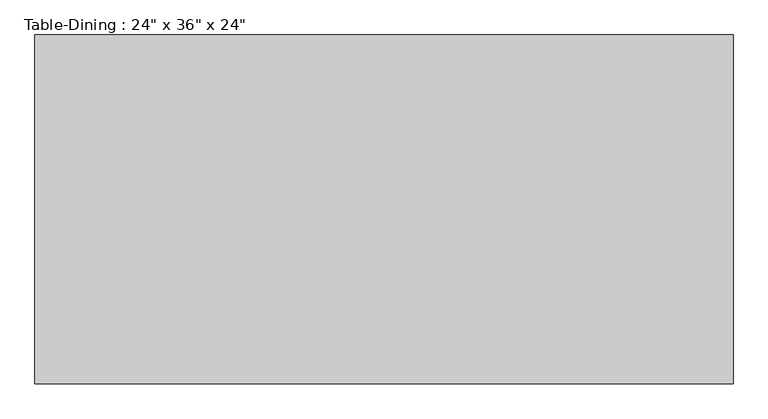
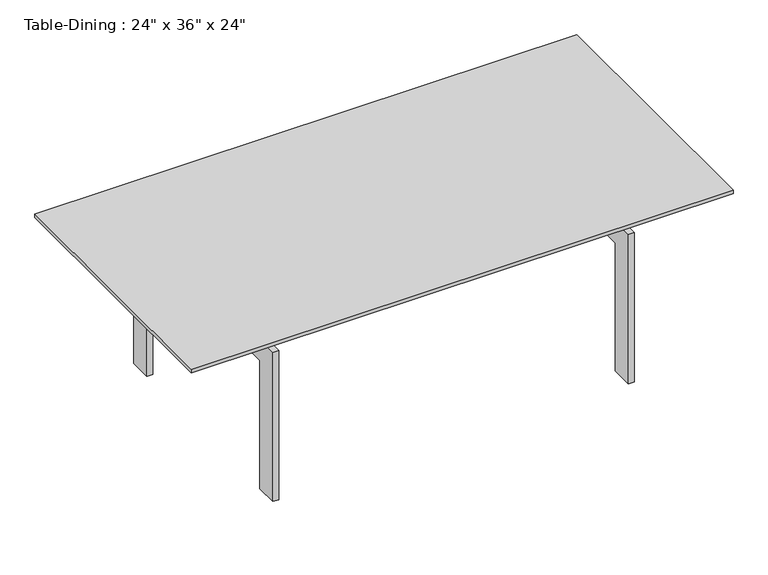
"""IFC4 building model written with IfcOpenShell, lengths in millimetres: furniture geometry."""

from ifc_helpers import new_model, si_unit, frame, origin, place, context, project, spatial, polyline, outline, extrude, source, transform, mapped, element, save


def furniture_5644571f(model_context):
    return source(origin(), model_context, "Body", "SweptSolid", [
        extrude(outline(polyline([(831.0657667, 297.7823857), (831.0657667, 272.3823857), (-794.5342333, 272.3823857), (-794.5342333, 297.7823857), (831.0657667, 297.7823857)])), frame((0.0, 0.0, 533.4), z_axis=(0.0, 0.0, 1.0), x_axis=(1.0, 0.0, 0.0)), (0.0, 0.0, 1.0), 63.5),
        extrude(outline(polyline([(831.0657667, -82.5889222), (831.0657667, -107.9889222), (-794.5342333, -107.9889222), (-794.5342333, -82.5889222), (831.0657667, -82.5889222)])), frame((0.0, 0.0, 533.4), z_axis=(0.0, 0.0, 1.0), x_axis=(1.0, 0.0, 0.0)), (0.0, 0.0, 1.0), 63.5),
        extrude(outline(polyline([(501.6110778, 0.0), (425.4110778, 0.0), (425.4110778, 457.2), (-234.9889222, 457.2), (-234.9889222, 0.0), (-311.1889222, 0.0), (-311.1889222, 533.4), (501.6110778, 533.4), (501.6110778, 0.0)])), frame((608.8157667, 0.0, 0.0), z_axis=(1.0, 0.0, 0.0), x_axis=(0.0, 1.0, 0.0)), (0.0, 0.0, 1.0), 19.05),
        extrude(outline(polyline([(501.6110778, 533.4), (501.6110778, 0.0), (425.4110778, 0.0), (425.4110778, 457.2), (-234.9889222, 457.2), (-234.9889222, 0.0), (-311.1889222, 0.0), (-311.1889222, 533.4), (501.6110778, 533.4)])), frame((-591.3342333, 0.0, 0.0), z_axis=(1.0, 0.0, 0.0), x_axis=(0.0, 1.0, 0.0)), (0.0, 0.0, 1.0), 19.05),
        extrude(outline(polyline([(932.6657667, 552.4110778), (932.6657667, -361.9889222), (-896.1342333, -361.9889222), (-896.1342333, 552.4110778), (932.6657667, 552.4110778)])), frame((0.0, 0.0, 596.9), z_axis=(0.0, 0.0, 1.0), x_axis=(1.0, 0.0, 0.0)), (0.0, 0.0, 1.0), 12.7),
    ])


if __name__ == "__main__":
    model = new_model("IFC4")
    model_context = context("Model", 3, world=origin())
    ifc_project = project(units=[si_unit("LENGTHUNIT", "METRE", prefix="MILLI")], contexts=[model_context])
    site = spatial("IfcSite", under=ifc_project)
    building = spatial("IfcBuilding", under=site)
    placement = place(None, origin())
    furniture_shape = furniture_5644571f(model_context)
    element("IfcFurniture", 1, ObjectType="Table-Dining : 24\" x 36\" x 24\"", at=placement, inside=building, context=model_context, shape_type="MappedRepresentation", body=[
        mapped(furniture_shape, transform((0.0, 0.0, 0.0), x_axis=(1.0, 0.0, 0.0), y_axis=(0.0, 1.0, 0.0), z_axis=(0.0, 0.0, 1.0))),
    ])
    save(model, "model.ifc")

# Revit data of these elements
# Type "Table-Dining : 24\" x 36\" x 24\""
#   Assembly Code = "E2020200"
#   Height = 2' - 0"
#   Length = 6' - 0"
#   Width = 3' - 0"
#   Base Material = Steel, Chrome Plated
#   Top Material = Glass - Clear, Grey
#   Default Elevation = 0
# Element 1 (IfcFurniture, "Table-Dining : 24\" x 36\" x 24\"")
#   Materials on its faces: "Steel, Chrome Plated", "Glass - Clear, Grey"
# Materials
#   "Steel, Chrome Plated": class "Metal", colour RGB 17 17 17, transparency 0, Description = "Chromiuim plated steel", Cost = 0
#   "Glass - Clear, Grey": class "Glass", colour RGB 252 255 255, transparency 0.64
